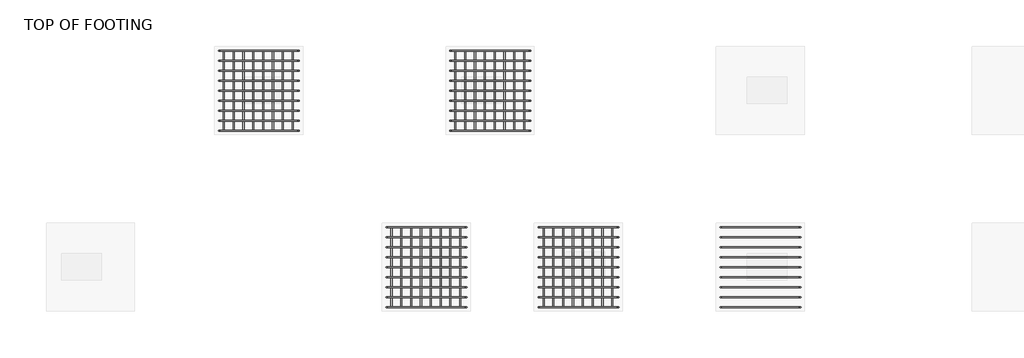
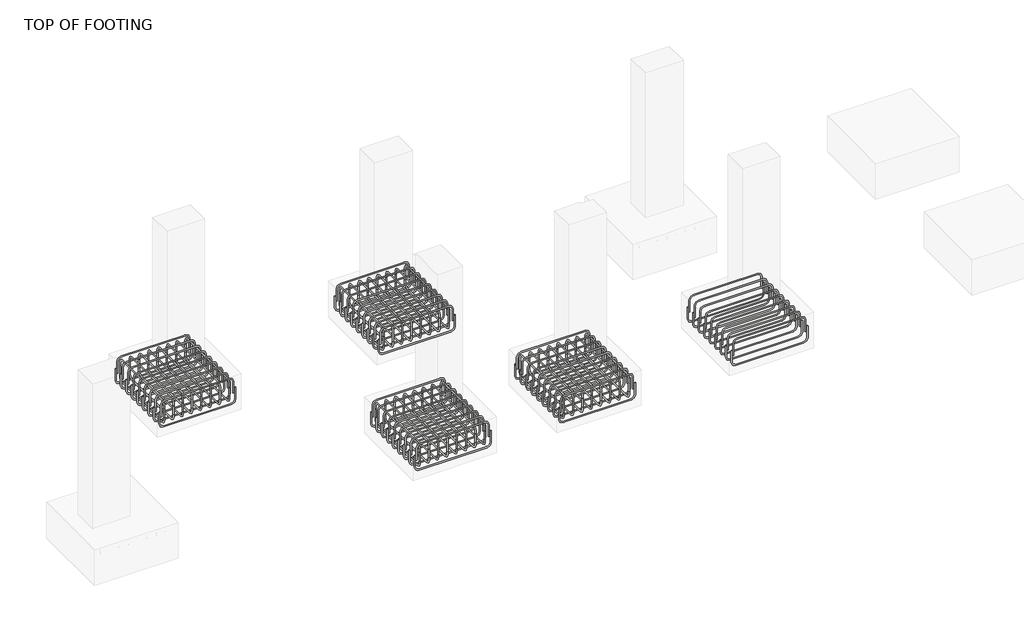
# One storey, part 7 of 20: 18 reinforcing bars.
"""IFC4 building model written with IfcOpenShell, lengths in millimetres."""

from ifc_helpers import new_model, si_unit, point, frame, origin, place, context, project, spatial, polyline, circle_curve, trimmed, segment, composite_curve, source, transform, mapped, element, save
from ifc_brep_helpers import swept_disk

model = new_model("IFC4")

# Units and contexts
model_context = context("Model", 3, world=origin())
ifc_project = project(units=[si_unit("LENGTHUNIT", "METRE", prefix="MILLI")], contexts=[model_context])

# Site, building, storey
site = spatial("IfcSite", under=ifc_project)
building = spatial("IfcBuilding", under=site)
storey = spatial("IfcBuildingStorey", under=building, Name="TOP OF FOOTING", Elevation=-1828.8)

# Reinforcing bars
placement = place(None, origin())
reinforcing_bar_shape = source(origin(), model_context, "Body", "SolidModel", [
    swept_disk(composite_curve([segment(polyline([(10322.7663908, -11304.2470059, -2006.6587682), (10322.7663908, -11304.2470059, -2153.9587682)]), True, "CONTINUOUS"), segment(trimmed(circle_curve(frame((10276.4163908, -11304.2470059, -2153.9587682), z_axis=(0.0, 1.0, 0.0), x_axis=(46.350000000000364, 0.0, 0.0)), 46.35), [point((10322.7663908, -11304.2470059, -2153.9587682))], [point((10276.4163908, -11304.2470059, -2200.3087682))], True, "CARTESIAN"), True, "CONTINUOUS"), segment(polyline([(10276.4163908, -11304.2470059, -2200.3087682), (9461.8163908, -11304.2470059, -2200.3087682)]), True, "CONTINUOUS"), segment(trimmed(circle_curve(frame((9461.8163908, -11304.2470059, -2153.9587682), z_axis=(0.0, 1.0, 0.0), x_axis=(0.0, 0.0, -46.34999999999991)), 46.35), [point((9461.8163908, -11304.2470059, -2200.3087682))], [point((9415.4663908, -11304.2470059, -2153.9587682))], True, "CARTESIAN"), True, "CONTINUOUS"), segment(polyline([(9415.4663908, -11304.2470059, -2153.9587682), (9415.4663908, -11304.2470059, -2006.6587682)]), True, "CONTINUOUS")], self_intersect=False), 6.35),
])
element("IfcReinforcingBar", 1, at=placement, inside=storey, context=model_context, shape_type="MappedRepresentation", body=[
    mapped(reinforcing_bar_shape, transform((0.0, 0.0, 0.0), x_axis=(1.0, 0.0, 0.0), y_axis=(0.0, 1.0, 0.0), z_axis=(0.0, 0.0, 1.0))),
    mapped(reinforcing_bar_shape, transform((0.0, -113.4125, 0.0), x_axis=(1.0, 0.0, 0.0), y_axis=(0.0, 1.0, 0.0), z_axis=(0.0, 0.0, 1.0))),
    mapped(reinforcing_bar_shape, transform((0.0, -226.825, 0.0), x_axis=(1.0, 0.0, 0.0), y_axis=(0.0, 1.0, 0.0), z_axis=(0.0, 0.0, 1.0))),
    mapped(reinforcing_bar_shape, transform((0.0, -340.2375, 0.0), x_axis=(1.0, 0.0, 0.0), y_axis=(0.0, 1.0, 0.0), z_axis=(0.0, 0.0, 1.0))),
    mapped(reinforcing_bar_shape, transform((0.0, -453.65, 0.0), x_axis=(1.0, 0.0, 0.0), y_axis=(0.0, 1.0, 0.0), z_axis=(0.0, 0.0, 1.0))),
    mapped(reinforcing_bar_shape, transform((0.0, -567.0625, 0.0), x_axis=(1.0, 0.0, 0.0), y_axis=(0.0, 1.0, 0.0), z_axis=(0.0, 0.0, 1.0))),
    mapped(reinforcing_bar_shape, transform((0.0, -680.475, 0.0), x_axis=(1.0, 0.0, 0.0), y_axis=(0.0, 1.0, 0.0), z_axis=(0.0, 0.0, 1.0))),
    mapped(reinforcing_bar_shape, transform((0.0, -793.8875, 0.0), x_axis=(1.0, 0.0, 0.0), y_axis=(0.0, 1.0, 0.0), z_axis=(0.0, 0.0, 1.0))),
    mapped(reinforcing_bar_shape, transform((0.0, -907.3, 0.0), x_axis=(1.0, 0.0, 0.0), y_axis=(0.0, 1.0, 0.0), z_axis=(0.0, 0.0, 1.0))),
])
reinforcing_bar_2_shape = source(origin(), model_context, "Body", "SolidModel", [
    swept_disk(composite_curve([segment(polyline([(9434.9405021, -11304.2470059, -2068.8), (9434.9405021, -11304.2470059, -1921.5)]), True, "CONTINUOUS"), segment(trimmed(circle_curve(frame((9481.2905021, -11304.2470059, -1921.5), z_axis=(0.0, 1.0, 0.0), x_axis=(-46.350000000000364, 0.0, 0.0)), 46.35), [point((9434.9405021, -11304.2470059, -1921.5))], [point((9481.2905021, -11304.2470059, -1875.15))], True, "CARTESIAN"), True, "CONTINUOUS"), segment(polyline([(9481.2905021, -11304.2470059, -1875.15), (10250.7539017, -11304.2470059, -1875.15)]), True, "CONTINUOUS"), segment(trimmed(circle_curve(frame((10250.7539017, -11304.2470059, -1921.5), z_axis=(0.0, 1.0, 0.0), x_axis=(0.0, 0.0, 46.34999999999991)), 46.35), [point((10250.7539017, -11304.2470059, -1875.15))], [point((10297.1039017, -11304.2470059, -1921.5))], True, "CARTESIAN"), True, "CONTINUOUS"), segment(polyline([(10297.1039017, -11304.2470059, -1921.5), (10297.1039017, -11304.2470059, -2068.8)]), True, "CONTINUOUS")], self_intersect=False), 6.35),
])
element("IfcReinforcingBar", 2, at=placement, inside=storey, context=model_context, shape_type="MappedRepresentation", body=[
    mapped(reinforcing_bar_2_shape, transform((0.0, 0.0, 0.0), x_axis=(1.0, 0.0, 0.0), y_axis=(0.0, 1.0, 0.0), z_axis=(0.0, 0.0, 1.0))),
    mapped(reinforcing_bar_2_shape, transform((0.0, -113.4125, 0.0), x_axis=(1.0, 0.0, 0.0), y_axis=(0.0, 1.0, 0.0), z_axis=(0.0, 0.0, 1.0))),
    mapped(reinforcing_bar_2_shape, transform((0.0, -226.825, 0.0), x_axis=(1.0, 0.0, 0.0), y_axis=(0.0, 1.0, 0.0), z_axis=(0.0, 0.0, 1.0))),
    mapped(reinforcing_bar_2_shape, transform((0.0, -340.2375, 0.0), x_axis=(1.0, 0.0, 0.0), y_axis=(0.0, 1.0, 0.0), z_axis=(0.0, 0.0, 1.0))),
    mapped(reinforcing_bar_2_shape, transform((0.0, -453.65, 0.0), x_axis=(1.0, 0.0, 0.0), y_axis=(0.0, 1.0, 0.0), z_axis=(0.0, 0.0, 1.0))),
    mapped(reinforcing_bar_2_shape, transform((0.0, -567.0625, 0.0), x_axis=(1.0, 0.0, 0.0), y_axis=(0.0, 1.0, 0.0), z_axis=(0.0, 0.0, 1.0))),
    mapped(reinforcing_bar_2_shape, transform((0.0, -680.475, 0.0), x_axis=(1.0, 0.0, 0.0), y_axis=(0.0, 1.0, 0.0), z_axis=(0.0, 0.0, 1.0))),
    mapped(reinforcing_bar_2_shape, transform((0.0, -793.8875, 0.0), x_axis=(1.0, 0.0, 0.0), y_axis=(0.0, 1.0, 0.0), z_axis=(0.0, 0.0, 1.0))),
    mapped(reinforcing_bar_2_shape, transform((0.0, -907.3, 0.0), x_axis=(1.0, 0.0, 0.0), y_axis=(0.0, 1.0, 0.0), z_axis=(0.0, 0.0, 1.0))),
])
reinforcing_bar_3_shape = source(origin(), model_context, "Body", "SolidModel", [
    swept_disk(composite_curve([segment(polyline([(7260.5179014, -9303.4578267, -2006.6587682), (7260.5179014, -9303.4578267, -2153.9587682)]), True, "CONTINUOUS"), segment(trimmed(circle_curve(frame((7214.1679014, -9303.4578267, -2153.9587682), z_axis=(0.0, 1.0, 0.0), x_axis=(46.349999999999454, 0.0, 0.0)), 46.35), [point((7260.5179014, -9303.4578267, -2153.9587682))], [point((7214.1679014, -9303.4578267, -2200.3087682))], True, "CARTESIAN"), True, "CONTINUOUS"), segment(polyline([(7214.1679014, -9303.4578267, -2200.3087682), (6399.5679014, -9303.4578267, -2200.3087682)]), True, "CONTINUOUS"), segment(trimmed(circle_curve(frame((6399.5679014, -9303.4578267, -2153.9587682), z_axis=(0.0, 1.0, 0.0), x_axis=(0.0, 0.0, -46.34999999999991)), 46.35), [point((6399.5679014, -9303.4578267, -2200.3087682))], [point((6353.2179014, -9303.4578267, -2153.9587682))], True, "CARTESIAN"), True, "CONTINUOUS"), segment(polyline([(6353.2179014, -9303.4578267, -2153.9587682), (6353.2179014, -9303.4578267, -2006.6587682)]), True, "CONTINUOUS")], self_intersect=False), 6.35),
])
element("IfcReinforcingBar", 3, at=placement, inside=storey, context=model_context, shape_type="MappedRepresentation", body=[
    mapped(reinforcing_bar_3_shape, transform((0.0, 0.0, 0.0), x_axis=(1.0, 0.0, 0.0), y_axis=(0.0, 1.0, 0.0), z_axis=(0.0, 0.0, 1.0))),
    mapped(reinforcing_bar_3_shape, transform((0.0, -113.4125, 0.0), x_axis=(1.0, 0.0, 0.0), y_axis=(0.0, 1.0, 0.0), z_axis=(0.0, 0.0, 1.0))),
    mapped(reinforcing_bar_3_shape, transform((0.0, -226.825, 0.0), x_axis=(1.0, 0.0, 0.0), y_axis=(0.0, 1.0, 0.0), z_axis=(0.0, 0.0, 1.0))),
    mapped(reinforcing_bar_3_shape, transform((0.0, -340.2375, 0.0), x_axis=(1.0, 0.0, 0.0), y_axis=(0.0, 1.0, 0.0), z_axis=(0.0, 0.0, 1.0))),
    mapped(reinforcing_bar_3_shape, transform((0.0, -453.65, 0.0), x_axis=(1.0, 0.0, 0.0), y_axis=(0.0, 1.0, 0.0), z_axis=(0.0, 0.0, 1.0))),
    mapped(reinforcing_bar_3_shape, transform((0.0, -567.0625, 0.0), x_axis=(1.0, 0.0, 0.0), y_axis=(0.0, 1.0, 0.0), z_axis=(0.0, 0.0, 1.0))),
    mapped(reinforcing_bar_3_shape, transform((0.0, -680.475, 0.0), x_axis=(1.0, 0.0, 0.0), y_axis=(0.0, 1.0, 0.0), z_axis=(0.0, 0.0, 1.0))),
    mapped(reinforcing_bar_3_shape, transform((0.0, -793.8875, 0.0), x_axis=(1.0, 0.0, 0.0), y_axis=(0.0, 1.0, 0.0), z_axis=(0.0, 0.0, 1.0))),
    mapped(reinforcing_bar_3_shape, transform((0.0, -907.3, 0.0), x_axis=(1.0, 0.0, 0.0), y_axis=(0.0, 1.0, 0.0), z_axis=(0.0, 0.0, 1.0))),
])
reinforcing_bar_4_shape = source(origin(), model_context, "Body", "SolidModel", [
    swept_disk(composite_curve([segment(polyline([(6372.6920127, -9303.4578267, -2068.8), (6372.6920127, -9303.4578267, -1921.5)]), True, "CONTINUOUS"), segment(trimmed(circle_curve(frame((6419.0420127, -9303.4578267, -1921.5), z_axis=(0.0, 1.0, 0.0), x_axis=(-46.349999999999454, 0.0, 0.0)), 46.35), [point((6372.6920127, -9303.4578267, -1921.5))], [point((6419.0420127, -9303.4578267, -1875.15))], True, "CARTESIAN"), True, "CONTINUOUS"), segment(polyline([(6419.0420127, -9303.4578267, -1875.15), (7188.5054124, -9303.4578267, -1875.15)]), True, "CONTINUOUS"), segment(trimmed(circle_curve(frame((7188.5054124, -9303.4578267, -1921.5), z_axis=(0.0, 1.0, 0.0), x_axis=(0.0, 0.0, 46.34999999999991)), 46.35), [point((7188.5054124, -9303.4578267, -1875.15))], [point((7234.8554124, -9303.4578267, -1921.5))], True, "CARTESIAN"), True, "CONTINUOUS"), segment(polyline([(7234.8554124, -9303.4578267, -1921.5), (7234.8554124, -9303.4578267, -2068.8)]), True, "CONTINUOUS")], self_intersect=False), 6.35),
])
element("IfcReinforcingBar", 4, at=placement, inside=storey, context=model_context, shape_type="MappedRepresentation", body=[
    mapped(reinforcing_bar_4_shape, transform((0.0, 0.0, 0.0), x_axis=(1.0, 0.0, 0.0), y_axis=(0.0, 1.0, 0.0), z_axis=(0.0, 0.0, 1.0))),
    mapped(reinforcing_bar_4_shape, transform((0.0, -113.4125, 0.0), x_axis=(1.0, 0.0, 0.0), y_axis=(0.0, 1.0, 0.0), z_axis=(0.0, 0.0, 1.0))),
    mapped(reinforcing_bar_4_shape, transform((0.0, -226.825, 0.0), x_axis=(1.0, 0.0, 0.0), y_axis=(0.0, 1.0, 0.0), z_axis=(0.0, 0.0, 1.0))),
    mapped(reinforcing_bar_4_shape, transform((0.0, -340.2375, 0.0), x_axis=(1.0, 0.0, 0.0), y_axis=(0.0, 1.0, 0.0), z_axis=(0.0, 0.0, 1.0))),
    mapped(reinforcing_bar_4_shape, transform((0.0, -453.65, 0.0), x_axis=(1.0, 0.0, 0.0), y_axis=(0.0, 1.0, 0.0), z_axis=(0.0, 0.0, 1.0))),
    mapped(reinforcing_bar_4_shape, transform((0.0, -567.0625, 0.0), x_axis=(1.0, 0.0, 0.0), y_axis=(0.0, 1.0, 0.0), z_axis=(0.0, 0.0, 1.0))),
    mapped(reinforcing_bar_4_shape, transform((0.0, -680.475, 0.0), x_axis=(1.0, 0.0, 0.0), y_axis=(0.0, 1.0, 0.0), z_axis=(0.0, 0.0, 1.0))),
    mapped(reinforcing_bar_4_shape, transform((0.0, -793.8875, 0.0), x_axis=(1.0, 0.0, 0.0), y_axis=(0.0, 1.0, 0.0), z_axis=(0.0, 0.0, 1.0))),
    mapped(reinforcing_bar_4_shape, transform((0.0, -907.3, 0.0), x_axis=(1.0, 0.0, 0.0), y_axis=(0.0, 1.0, 0.0), z_axis=(0.0, 0.0, 1.0))),
])
reinforcing_bar_5_shape = source(origin(), model_context, "Body", "SolidModel", [
    swept_disk(composite_curve([segment(polyline([(7189.02094, -9303.4578267, -2086.1951968), (7189.02094, -9303.4578267, -1938.8951968)]), True, "CONTINUOUS"), segment(trimmed(circle_curve(frame((7189.02094, -9349.8078267, -1938.8951968), z_axis=(1.0, 0.0, 0.0), x_axis=(0.0, 46.350000000000364, 0.0)), 46.35), [point((7189.02094, -9303.4578267, -1938.8951968))], [point((7189.02094, -9349.8078267, -1892.5451968))], True, "CARTESIAN"), True, "CONTINUOUS"), segment(polyline([(7189.02094, -9349.8078267, -1892.5451968), (7189.02094, -10164.4078267, -1892.5451968)]), True, "CONTINUOUS"), segment(trimmed(circle_curve(frame((7189.02094, -10164.4078267, -1938.8951968), z_axis=(1.0, 0.0, 0.0), x_axis=(0.0, 0.0, 46.34999999999991)), 46.35), [point((7189.02094, -10164.4078267, -1892.5451968))], [point((7189.02094, -10210.7578267, -1938.8951968))], True, "CARTESIAN"), True, "CONTINUOUS"), segment(polyline([(7189.02094, -10210.7578267, -1938.8951968), (7189.02094, -10210.7578267, -2086.1951968)]), True, "CONTINUOUS")], self_intersect=False), 6.35),
])
element("IfcReinforcingBar", 5, at=placement, inside=storey, context=model_context, shape_type="MappedRepresentation", body=[
    mapped(reinforcing_bar_5_shape, transform((0.0, 0.0, 0.0), x_axis=(1.0, 0.0, 0.0), y_axis=(0.0, 1.0, 0.0), z_axis=(0.0, 0.0, 1.0))),
    mapped(reinforcing_bar_5_shape, transform((-111.2862402, 0.0, 0.0), x_axis=(1.0, 0.0, 0.0), y_axis=(0.0, 1.0, 0.0), z_axis=(0.0, 0.0, 1.0))),
    mapped(reinforcing_bar_5_shape, transform((-222.5724804, 0.0, 0.0), x_axis=(1.0, 0.0, 0.0), y_axis=(0.0, 1.0, 0.0), z_axis=(0.0, 0.0, 1.0))),
    mapped(reinforcing_bar_5_shape, transform((-333.8587205, 0.0, 0.0), x_axis=(1.0, 0.0, 0.0), y_axis=(0.0, 1.0, 0.0), z_axis=(0.0, 0.0, 1.0))),
    mapped(reinforcing_bar_5_shape, transform((-445.1449607, 0.0, 0.0), x_axis=(1.0, 0.0, 0.0), y_axis=(0.0, 1.0, 0.0), z_axis=(0.0, 0.0, 1.0))),
    mapped(reinforcing_bar_5_shape, transform((-556.4312009, 0.0, 0.0), x_axis=(1.0, 0.0, 0.0), y_axis=(0.0, 1.0, 0.0), z_axis=(0.0, 0.0, 1.0))),
    mapped(reinforcing_bar_5_shape, transform((-667.7174411, 0.0, 0.0), x_axis=(1.0, 0.0, 0.0), y_axis=(0.0, 1.0, 0.0), z_axis=(0.0, 0.0, 1.0))),
    mapped(reinforcing_bar_5_shape, transform((-779.0036813, 0.0, 0.0), x_axis=(1.0, 0.0, 0.0), y_axis=(0.0, 1.0, 0.0), z_axis=(0.0, 0.0, 1.0))),
])
reinforcing_bar_6_shape = source(origin(), model_context, "Body", "SolidModel", [
    swept_disk(composite_curve([segment(polyline([(6410.0172587, -9303.4578267, -1979.1645013), (6410.0172587, -9303.4578267, -2126.4645013)]), True, "CONTINUOUS"), segment(trimmed(circle_curve(frame((6410.0172587, -9349.8078267, -2126.4645013), z_axis=(-1.0, 0.0, 0.0), x_axis=(0.0, 46.350000000000364, 0.0)), 46.35), [point((6410.0172587, -9303.4578267, -2126.4645013))], [point((6410.0172587, -9349.8078267, -2172.8145013))], True, "CARTESIAN"), True, "CONTINUOUS"), segment(polyline([(6410.0172587, -9349.8078267, -2172.8145013), (6410.0172587, -10164.4078267, -2172.8145013)]), True, "CONTINUOUS"), segment(trimmed(circle_curve(frame((6410.0172587, -10164.4078267, -2126.4645013), z_axis=(-1.0, 0.0, 0.0), x_axis=(0.0, 0.0, -46.34999999999991)), 46.35), [point((6410.0172587, -10164.4078267, -2172.8145013))], [point((6410.0172587, -10210.7578267, -2126.4645013))], True, "CARTESIAN"), True, "CONTINUOUS"), segment(polyline([(6410.0172587, -10210.7578267, -2126.4645013), (6410.0172587, -10210.7578267, -1979.1645013)]), True, "CONTINUOUS")], self_intersect=False), 6.35),
])
element("IfcReinforcingBar", 6, at=placement, inside=storey, context=model_context, shape_type="MappedRepresentation", body=[
    mapped(reinforcing_bar_6_shape, transform((0.0, 0.0, 0.0), x_axis=(1.0, 0.0, 0.0), y_axis=(0.0, 1.0, 0.0), z_axis=(0.0, 0.0, 1.0))),
    mapped(reinforcing_bar_6_shape, transform((111.2862402, 0.0, 0.0), x_axis=(1.0, 0.0, 0.0), y_axis=(0.0, 1.0, 0.0), z_axis=(0.0, 0.0, 1.0))),
    mapped(reinforcing_bar_6_shape, transform((222.5724804, 0.0, 0.0), x_axis=(1.0, 0.0, 0.0), y_axis=(0.0, 1.0, 0.0), z_axis=(0.0, 0.0, 1.0))),
    mapped(reinforcing_bar_6_shape, transform((333.8587205, 0.0, 0.0), x_axis=(1.0, 0.0, 0.0), y_axis=(0.0, 1.0, 0.0), z_axis=(0.0, 0.0, 1.0))),
    mapped(reinforcing_bar_6_shape, transform((445.1449607, 0.0, 0.0), x_axis=(1.0, 0.0, 0.0), y_axis=(0.0, 1.0, 0.0), z_axis=(0.0, 0.0, 1.0))),
    mapped(reinforcing_bar_6_shape, transform((556.4312009, 0.0, 0.0), x_axis=(1.0, 0.0, 0.0), y_axis=(0.0, 1.0, 0.0), z_axis=(0.0, 0.0, 1.0))),
    mapped(reinforcing_bar_6_shape, transform((667.7174411, 0.0, 0.0), x_axis=(1.0, 0.0, 0.0), y_axis=(0.0, 1.0, 0.0), z_axis=(0.0, 0.0, 1.0))),
    mapped(reinforcing_bar_6_shape, transform((779.0036813, 0.0, 0.0), x_axis=(1.0, 0.0, 0.0), y_axis=(0.0, 1.0, 0.0), z_axis=(0.0, 0.0, 1.0))),
])
reinforcing_bar_7_shape = source(origin(), model_context, "Body", "SolidModel", [
    swept_disk(composite_curve([segment(polyline([(6536.1748054, -11304.2470059, -2006.6587682), (6536.1748054, -11304.2470059, -2153.9587682)]), True, "CONTINUOUS"), segment(trimmed(circle_curve(frame((6489.8248054, -11304.2470059, -2153.9587682), z_axis=(0.0, 1.0, 0.0), x_axis=(46.350000000000364, 0.0, 0.0)), 46.35), [point((6536.1748054, -11304.2470059, -2153.9587682))], [point((6489.8248054, -11304.2470059, -2200.3087682))], True, "CARTESIAN"), True, "CONTINUOUS"), segment(polyline([(6489.8248054, -11304.2470059, -2200.3087682), (5675.2248054, -11304.2470059, -2200.3087682)]), True, "CONTINUOUS"), segment(trimmed(circle_curve(frame((5675.2248054, -11304.2470059, -2153.9587682), z_axis=(0.0, 1.0, 0.0), x_axis=(0.0, 0.0, -46.34999999999991)), 46.35), [point((5675.2248054, -11304.2470059, -2200.3087682))], [point((5628.8748054, -11304.2470059, -2153.9587682))], True, "CARTESIAN"), True, "CONTINUOUS"), segment(polyline([(5628.8748054, -11304.2470059, -2153.9587682), (5628.8748054, -11304.2470059, -2006.6587682)]), True, "CONTINUOUS")], self_intersect=False), 6.35),
])
element("IfcReinforcingBar", 7, at=placement, inside=storey, context=model_context, shape_type="MappedRepresentation", body=[
    mapped(reinforcing_bar_7_shape, transform((0.0, 0.0, 0.0), x_axis=(1.0, 0.0, 0.0), y_axis=(0.0, 1.0, 0.0), z_axis=(0.0, 0.0, 1.0))),
    mapped(reinforcing_bar_7_shape, transform((0.0, -113.4125, 0.0), x_axis=(1.0, 0.0, 0.0), y_axis=(0.0, 1.0, 0.0), z_axis=(0.0, 0.0, 1.0))),
    mapped(reinforcing_bar_7_shape, transform((0.0, -226.825, 0.0), x_axis=(1.0, 0.0, 0.0), y_axis=(0.0, 1.0, 0.0), z_axis=(0.0, 0.0, 1.0))),
    mapped(reinforcing_bar_7_shape, transform((0.0, -340.2375, 0.0), x_axis=(1.0, 0.0, 0.0), y_axis=(0.0, 1.0, 0.0), z_axis=(0.0, 0.0, 1.0))),
    mapped(reinforcing_bar_7_shape, transform((0.0, -453.65, 0.0), x_axis=(1.0, 0.0, 0.0), y_axis=(0.0, 1.0, 0.0), z_axis=(0.0, 0.0, 1.0))),
    mapped(reinforcing_bar_7_shape, transform((0.0, -567.0625, 0.0), x_axis=(1.0, 0.0, 0.0), y_axis=(0.0, 1.0, 0.0), z_axis=(0.0, 0.0, 1.0))),
    mapped(reinforcing_bar_7_shape, transform((0.0, -680.475, 0.0), x_axis=(1.0, 0.0, 0.0), y_axis=(0.0, 1.0, 0.0), z_axis=(0.0, 0.0, 1.0))),
    mapped(reinforcing_bar_7_shape, transform((0.0, -793.8875, 0.0), x_axis=(1.0, 0.0, 0.0), y_axis=(0.0, 1.0, 0.0), z_axis=(0.0, 0.0, 1.0))),
    mapped(reinforcing_bar_7_shape, transform((0.0, -907.3, 0.0), x_axis=(1.0, 0.0, 0.0), y_axis=(0.0, 1.0, 0.0), z_axis=(0.0, 0.0, 1.0))),
])
reinforcing_bar_8_shape = source(origin(), model_context, "Body", "SolidModel", [
    swept_disk(composite_curve([segment(polyline([(5648.3489167, -11304.2470059, -2068.8), (5648.3489167, -11304.2470059, -1921.5)]), True, "CONTINUOUS"), segment(trimmed(circle_curve(frame((5694.6989167, -11304.2470059, -1921.5), z_axis=(0.0, 1.0, 0.0), x_axis=(-46.350000000000364, 0.0, 0.0)), 46.35), [point((5648.3489167, -11304.2470059, -1921.5))], [point((5694.6989167, -11304.2470059, -1875.15))], True, "CARTESIAN"), True, "CONTINUOUS"), segment(polyline([(5694.6989167, -11304.2470059, -1875.15), (6464.1623164, -11304.2470059, -1875.15)]), True, "CONTINUOUS"), segment(trimmed(circle_curve(frame((6464.1623164, -11304.2470059, -1921.5), z_axis=(0.0, 1.0, 0.0), x_axis=(0.0, 0.0, 46.34999999999991)), 46.35), [point((6464.1623164, -11304.2470059, -1875.15))], [point((6510.5123164, -11304.2470059, -1921.5))], True, "CARTESIAN"), True, "CONTINUOUS"), segment(polyline([(6510.5123164, -11304.2470059, -1921.5), (6510.5123164, -11304.2470059, -2068.8)]), True, "CONTINUOUS")], self_intersect=False), 6.35),
])
element("IfcReinforcingBar", 8, at=placement, inside=storey, context=model_context, shape_type="MappedRepresentation", body=[
    mapped(reinforcing_bar_8_shape, transform((0.0, 0.0, 0.0), x_axis=(1.0, 0.0, 0.0), y_axis=(0.0, 1.0, 0.0), z_axis=(0.0, 0.0, 1.0))),
    mapped(reinforcing_bar_8_shape, transform((0.0, -113.4125, 0.0), x_axis=(1.0, 0.0, 0.0), y_axis=(0.0, 1.0, 0.0), z_axis=(0.0, 0.0, 1.0))),
    mapped(reinforcing_bar_8_shape, transform((0.0, -226.825, 0.0), x_axis=(1.0, 0.0, 0.0), y_axis=(0.0, 1.0, 0.0), z_axis=(0.0, 0.0, 1.0))),
    mapped(reinforcing_bar_8_shape, transform((0.0, -340.2375, 0.0), x_axis=(1.0, 0.0, 0.0), y_axis=(0.0, 1.0, 0.0), z_axis=(0.0, 0.0, 1.0))),
    mapped(reinforcing_bar_8_shape, transform((0.0, -453.65, 0.0), x_axis=(1.0, 0.0, 0.0), y_axis=(0.0, 1.0, 0.0), z_axis=(0.0, 0.0, 1.0))),
    mapped(reinforcing_bar_8_shape, transform((0.0, -567.0625, 0.0), x_axis=(1.0, 0.0, 0.0), y_axis=(0.0, 1.0, 0.0), z_axis=(0.0, 0.0, 1.0))),
    mapped(reinforcing_bar_8_shape, transform((0.0, -680.475, 0.0), x_axis=(1.0, 0.0, 0.0), y_axis=(0.0, 1.0, 0.0), z_axis=(0.0, 0.0, 1.0))),
    mapped(reinforcing_bar_8_shape, transform((0.0, -793.8875, 0.0), x_axis=(1.0, 0.0, 0.0), y_axis=(0.0, 1.0, 0.0), z_axis=(0.0, 0.0, 1.0))),
    mapped(reinforcing_bar_8_shape, transform((0.0, -907.3, 0.0), x_axis=(1.0, 0.0, 0.0), y_axis=(0.0, 1.0, 0.0), z_axis=(0.0, 0.0, 1.0))),
])
reinforcing_bar_9_shape = source(origin(), model_context, "Body", "SolidModel", [
    swept_disk(composite_curve([segment(polyline([(6464.677844, -11304.2470059, -2086.1951968), (6464.677844, -11304.2470059, -1938.8951968)]), True, "CONTINUOUS"), segment(trimmed(circle_curve(frame((6464.677844, -11350.5970059, -1938.8951968), z_axis=(1.0, 0.0, 0.0), x_axis=(0.0, 46.349999999998545, 0.0)), 46.35), [point((6464.677844, -11304.2470059, -1938.8951968))], [point((6464.677844, -11350.5970059, -1892.5451968))], True, "CARTESIAN"), True, "CONTINUOUS"), segment(polyline([(6464.677844, -11350.5970059, -1892.5451968), (6464.677844, -12165.1970059, -1892.5451968)]), True, "CONTINUOUS"), segment(trimmed(circle_curve(frame((6464.677844, -12165.1970059, -1938.8951968), z_axis=(1.0, 0.0, 0.0), x_axis=(0.0, 0.0, 46.34999999999991)), 46.35), [point((6464.677844, -12165.1970059, -1892.5451968))], [point((6464.677844, -12211.5470059, -1938.8951968))], True, "CARTESIAN"), True, "CONTINUOUS"), segment(polyline([(6464.677844, -12211.5470059, -1938.8951968), (6464.677844, -12211.5470059, -2086.1951968)]), True, "CONTINUOUS")], self_intersect=False), 6.35),
])
element("IfcReinforcingBar", 9, at=placement, inside=storey, context=model_context, shape_type="MappedRepresentation", body=[
    mapped(reinforcing_bar_9_shape, transform((0.0, 0.0, 0.0), x_axis=(1.0, 0.0, 0.0), y_axis=(0.0, 1.0, 0.0), z_axis=(0.0, 0.0, 1.0))),
    mapped(reinforcing_bar_9_shape, transform((-111.2862402, 0.0, 0.0), x_axis=(1.0, 0.0, 0.0), y_axis=(0.0, 1.0, 0.0), z_axis=(0.0, 0.0, 1.0))),
    mapped(reinforcing_bar_9_shape, transform((-222.5724804, 0.0, 0.0), x_axis=(1.0, 0.0, 0.0), y_axis=(0.0, 1.0, 0.0), z_axis=(0.0, 0.0, 1.0))),
    mapped(reinforcing_bar_9_shape, transform((-333.8587205, 0.0, 0.0), x_axis=(1.0, 0.0, 0.0), y_axis=(0.0, 1.0, 0.0), z_axis=(0.0, 0.0, 1.0))),
    mapped(reinforcing_bar_9_shape, transform((-445.1449607, 0.0, 0.0), x_axis=(1.0, 0.0, 0.0), y_axis=(0.0, 1.0, 0.0), z_axis=(0.0, 0.0, 1.0))),
    mapped(reinforcing_bar_9_shape, transform((-556.4312009, 0.0, 0.0), x_axis=(1.0, 0.0, 0.0), y_axis=(0.0, 1.0, 0.0), z_axis=(0.0, 0.0, 1.0))),
    mapped(reinforcing_bar_9_shape, transform((-667.7174411, 0.0, 0.0), x_axis=(1.0, 0.0, 0.0), y_axis=(0.0, 1.0, 0.0), z_axis=(0.0, 0.0, 1.0))),
    mapped(reinforcing_bar_9_shape, transform((-779.0036813, 0.0, 0.0), x_axis=(1.0, 0.0, 0.0), y_axis=(0.0, 1.0, 0.0), z_axis=(0.0, 0.0, 1.0))),
])
reinforcing_bar_10_shape = source(origin(), model_context, "Body", "SolidModel", [
    swept_disk(composite_curve([segment(polyline([(5685.6741627, -11304.2470059, -1979.1645013), (5685.6741627, -11304.2470059, -2126.4645013)]), True, "CONTINUOUS"), segment(trimmed(circle_curve(frame((5685.6741627, -11350.5970059, -2126.4645013), z_axis=(-1.0, 0.0, 0.0), x_axis=(0.0, 46.349999999998545, 0.0)), 46.35), [point((5685.6741627, -11304.2470059, -2126.4645013))], [point((5685.6741627, -11350.5970059, -2172.8145013))], True, "CARTESIAN"), True, "CONTINUOUS"), segment(polyline([(5685.6741627, -11350.5970059, -2172.8145013), (5685.6741627, -12165.1970059, -2172.8145013)]), True, "CONTINUOUS"), segment(trimmed(circle_curve(frame((5685.6741627, -12165.1970059, -2126.4645013), z_axis=(-1.0, 0.0, 0.0), x_axis=(0.0, 0.0, -46.34999999999991)), 46.35), [point((5685.6741627, -12165.1970059, -2172.8145013))], [point((5685.6741627, -12211.5470059, -2126.4645013))], True, "CARTESIAN"), True, "CONTINUOUS"), segment(polyline([(5685.6741627, -12211.5470059, -2126.4645013), (5685.6741627, -12211.5470059, -1979.1645013)]), True, "CONTINUOUS")], self_intersect=False), 6.35),
])
element("IfcReinforcingBar", 10, at=placement, inside=storey, context=model_context, shape_type="MappedRepresentation", body=[
    mapped(reinforcing_bar_10_shape, transform((0.0, 0.0, 0.0), x_axis=(1.0, 0.0, 0.0), y_axis=(0.0, 1.0, 0.0), z_axis=(0.0, 0.0, 1.0))),
    mapped(reinforcing_bar_10_shape, transform((111.2862402, 0.0, 0.0), x_axis=(1.0, 0.0, 0.0), y_axis=(0.0, 1.0, 0.0), z_axis=(0.0, 0.0, 1.0))),
    mapped(reinforcing_bar_10_shape, transform((222.5724804, 0.0, 0.0), x_axis=(1.0, 0.0, 0.0), y_axis=(0.0, 1.0, 0.0), z_axis=(0.0, 0.0, 1.0))),
    mapped(reinforcing_bar_10_shape, transform((333.8587205, 0.0, 0.0), x_axis=(1.0, 0.0, 0.0), y_axis=(0.0, 1.0, 0.0), z_axis=(0.0, 0.0, 1.0))),
    mapped(reinforcing_bar_10_shape, transform((445.1449607, 0.0, 0.0), x_axis=(1.0, 0.0, 0.0), y_axis=(0.0, 1.0, 0.0), z_axis=(0.0, 0.0, 1.0))),
    mapped(reinforcing_bar_10_shape, transform((556.4312009, 0.0, 0.0), x_axis=(1.0, 0.0, 0.0), y_axis=(0.0, 1.0, 0.0), z_axis=(0.0, 0.0, 1.0))),
    mapped(reinforcing_bar_10_shape, transform((667.7174411, 0.0, 0.0), x_axis=(1.0, 0.0, 0.0), y_axis=(0.0, 1.0, 0.0), z_axis=(0.0, 0.0, 1.0))),
    mapped(reinforcing_bar_10_shape, transform((779.0036813, 0.0, 0.0), x_axis=(1.0, 0.0, 0.0), y_axis=(0.0, 1.0, 0.0), z_axis=(0.0, 0.0, 1.0))),
])
reinforcing_bar_11_shape = source(origin(), model_context, "Body", "SolidModel", [
    swept_disk(composite_curve([segment(polyline([(8260.5179014, -11304.2470059, -2006.6587682), (8260.5179014, -11304.2470059, -2153.9587682)]), True, "CONTINUOUS"), segment(trimmed(circle_curve(frame((8214.1679014, -11304.2470059, -2153.9587682), z_axis=(0.0, 1.0, 0.0), x_axis=(46.350000000000364, 0.0, 0.0)), 46.35), [point((8260.5179014, -11304.2470059, -2153.9587682))], [point((8214.1679014, -11304.2470059, -2200.3087682))], True, "CARTESIAN"), True, "CONTINUOUS"), segment(polyline([(8214.1679014, -11304.2470059, -2200.3087682), (7399.5679014, -11304.2470059, -2200.3087682)]), True, "CONTINUOUS"), segment(trimmed(circle_curve(frame((7399.5679014, -11304.2470059, -2153.9587682), z_axis=(0.0, 1.0, 0.0), x_axis=(0.0, 0.0, -46.34999999999991)), 46.35), [point((7399.5679014, -11304.2470059, -2200.3087682))], [point((7353.2179014, -11304.2470059, -2153.9587682))], True, "CARTESIAN"), True, "CONTINUOUS"), segment(polyline([(7353.2179014, -11304.2470059, -2153.9587682), (7353.2179014, -11304.2470059, -2006.6587682)]), True, "CONTINUOUS")], self_intersect=False), 6.35),
])
element("IfcReinforcingBar", 11, at=placement, inside=storey, context=model_context, shape_type="MappedRepresentation", body=[
    mapped(reinforcing_bar_11_shape, transform((0.0, 0.0, 0.0), x_axis=(1.0, 0.0, 0.0), y_axis=(0.0, 1.0, 0.0), z_axis=(0.0, 0.0, 1.0))),
    mapped(reinforcing_bar_11_shape, transform((0.0, -113.4125, 0.0), x_axis=(1.0, 0.0, 0.0), y_axis=(0.0, 1.0, 0.0), z_axis=(0.0, 0.0, 1.0))),
    mapped(reinforcing_bar_11_shape, transform((0.0, -226.825, 0.0), x_axis=(1.0, 0.0, 0.0), y_axis=(0.0, 1.0, 0.0), z_axis=(0.0, 0.0, 1.0))),
    mapped(reinforcing_bar_11_shape, transform((0.0, -340.2375, 0.0), x_axis=(1.0, 0.0, 0.0), y_axis=(0.0, 1.0, 0.0), z_axis=(0.0, 0.0, 1.0))),
    mapped(reinforcing_bar_11_shape, transform((0.0, -453.65, 0.0), x_axis=(1.0, 0.0, 0.0), y_axis=(0.0, 1.0, 0.0), z_axis=(0.0, 0.0, 1.0))),
    mapped(reinforcing_bar_11_shape, transform((0.0, -567.0625, 0.0), x_axis=(1.0, 0.0, 0.0), y_axis=(0.0, 1.0, 0.0), z_axis=(0.0, 0.0, 1.0))),
    mapped(reinforcing_bar_11_shape, transform((0.0, -680.475, 0.0), x_axis=(1.0, 0.0, 0.0), y_axis=(0.0, 1.0, 0.0), z_axis=(0.0, 0.0, 1.0))),
    mapped(reinforcing_bar_11_shape, transform((0.0, -793.8875, 0.0), x_axis=(1.0, 0.0, 0.0), y_axis=(0.0, 1.0, 0.0), z_axis=(0.0, 0.0, 1.0))),
    mapped(reinforcing_bar_11_shape, transform((0.0, -907.3, 0.0), x_axis=(1.0, 0.0, 0.0), y_axis=(0.0, 1.0, 0.0), z_axis=(0.0, 0.0, 1.0))),
])
reinforcing_bar_12_shape = source(origin(), model_context, "Body", "SolidModel", [
    swept_disk(composite_curve([segment(polyline([(7372.6920127, -11304.2470059, -2068.8), (7372.6920127, -11304.2470059, -1921.5)]), True, "CONTINUOUS"), segment(trimmed(circle_curve(frame((7419.0420127, -11304.2470059, -1921.5), z_axis=(0.0, 1.0, 0.0), x_axis=(-46.349999999999454, 0.0, 0.0)), 46.35), [point((7372.6920127, -11304.2470059, -1921.5))], [point((7419.0420127, -11304.2470059, -1875.15))], True, "CARTESIAN"), True, "CONTINUOUS"), segment(polyline([(7419.0420127, -11304.2470059, -1875.15), (8188.5054124, -11304.2470059, -1875.15)]), True, "CONTINUOUS"), segment(trimmed(circle_curve(frame((8188.5054124, -11304.2470059, -1921.5), z_axis=(0.0, 1.0, 0.0), x_axis=(0.0, 0.0, 46.34999999999991)), 46.35), [point((8188.5054124, -11304.2470059, -1875.15))], [point((8234.8554124, -11304.2470059, -1921.5))], True, "CARTESIAN"), True, "CONTINUOUS"), segment(polyline([(8234.8554124, -11304.2470059, -1921.5), (8234.8554124, -11304.2470059, -2068.8)]), True, "CONTINUOUS")], self_intersect=False), 6.35),
])
element("IfcReinforcingBar", 12, at=placement, inside=storey, context=model_context, shape_type="MappedRepresentation", body=[
    mapped(reinforcing_bar_12_shape, transform((0.0, 0.0, 0.0), x_axis=(1.0, 0.0, 0.0), y_axis=(0.0, 1.0, 0.0), z_axis=(0.0, 0.0, 1.0))),
    mapped(reinforcing_bar_12_shape, transform((0.0, -113.4125, 0.0), x_axis=(1.0, 0.0, 0.0), y_axis=(0.0, 1.0, 0.0), z_axis=(0.0, 0.0, 1.0))),
    mapped(reinforcing_bar_12_shape, transform((0.0, -226.825, 0.0), x_axis=(1.0, 0.0, 0.0), y_axis=(0.0, 1.0, 0.0), z_axis=(0.0, 0.0, 1.0))),
    mapped(reinforcing_bar_12_shape, transform((0.0, -340.2375, 0.0), x_axis=(1.0, 0.0, 0.0), y_axis=(0.0, 1.0, 0.0), z_axis=(0.0, 0.0, 1.0))),
    mapped(reinforcing_bar_12_shape, transform((0.0, -453.65, 0.0), x_axis=(1.0, 0.0, 0.0), y_axis=(0.0, 1.0, 0.0), z_axis=(0.0, 0.0, 1.0))),
    mapped(reinforcing_bar_12_shape, transform((0.0, -567.0625, 0.0), x_axis=(1.0, 0.0, 0.0), y_axis=(0.0, 1.0, 0.0), z_axis=(0.0, 0.0, 1.0))),
    mapped(reinforcing_bar_12_shape, transform((0.0, -680.475, 0.0), x_axis=(1.0, 0.0, 0.0), y_axis=(0.0, 1.0, 0.0), z_axis=(0.0, 0.0, 1.0))),
    mapped(reinforcing_bar_12_shape, transform((0.0, -793.8875, 0.0), x_axis=(1.0, 0.0, 0.0), y_axis=(0.0, 1.0, 0.0), z_axis=(0.0, 0.0, 1.0))),
    mapped(reinforcing_bar_12_shape, transform((0.0, -907.3, 0.0), x_axis=(1.0, 0.0, 0.0), y_axis=(0.0, 1.0, 0.0), z_axis=(0.0, 0.0, 1.0))),
])
reinforcing_bar_13_shape = source(origin(), model_context, "Body", "SolidModel", [
    swept_disk(composite_curve([segment(polyline([(8189.02094, -11304.2470059, -2086.1951968), (8189.02094, -11304.2470059, -1938.8951968)]), True, "CONTINUOUS"), segment(trimmed(circle_curve(frame((8189.02094, -11350.5970059, -1938.8951968), z_axis=(1.0, 0.0, 0.0), x_axis=(0.0, 46.349999999998545, 0.0)), 46.35), [point((8189.02094, -11304.2470059, -1938.8951968))], [point((8189.02094, -11350.5970059, -1892.5451968))], True, "CARTESIAN"), True, "CONTINUOUS"), segment(polyline([(8189.02094, -11350.5970059, -1892.5451968), (8189.02094, -12165.1970059, -1892.5451968)]), True, "CONTINUOUS"), segment(trimmed(circle_curve(frame((8189.02094, -12165.1970059, -1938.8951968), z_axis=(1.0, 0.0, 0.0), x_axis=(0.0, 0.0, 46.34999999999991)), 46.35), [point((8189.02094, -12165.1970059, -1892.5451968))], [point((8189.02094, -12211.5470059, -1938.8951968))], True, "CARTESIAN"), True, "CONTINUOUS"), segment(polyline([(8189.02094, -12211.5470059, -1938.8951968), (8189.02094, -12211.5470059, -2086.1951968)]), True, "CONTINUOUS")], self_intersect=False), 6.35),
])
element("IfcReinforcingBar", 13, at=placement, inside=storey, context=model_context, shape_type="MappedRepresentation", body=[
    mapped(reinforcing_bar_13_shape, transform((0.0, 0.0, 0.0), x_axis=(1.0, 0.0, 0.0), y_axis=(0.0, 1.0, 0.0), z_axis=(0.0, 0.0, 1.0))),
    mapped(reinforcing_bar_13_shape, transform((-111.2862402, 0.0, 0.0), x_axis=(1.0, 0.0, 0.0), y_axis=(0.0, 1.0, 0.0), z_axis=(0.0, 0.0, 1.0))),
    mapped(reinforcing_bar_13_shape, transform((-222.5724804, 0.0, 0.0), x_axis=(1.0, 0.0, 0.0), y_axis=(0.0, 1.0, 0.0), z_axis=(0.0, 0.0, 1.0))),
    mapped(reinforcing_bar_13_shape, transform((-333.8587205, 0.0, 0.0), x_axis=(1.0, 0.0, 0.0), y_axis=(0.0, 1.0, 0.0), z_axis=(0.0, 0.0, 1.0))),
    mapped(reinforcing_bar_13_shape, transform((-445.1449607, 0.0, 0.0), x_axis=(1.0, 0.0, 0.0), y_axis=(0.0, 1.0, 0.0), z_axis=(0.0, 0.0, 1.0))),
    mapped(reinforcing_bar_13_shape, transform((-556.4312009, 0.0, 0.0), x_axis=(1.0, 0.0, 0.0), y_axis=(0.0, 1.0, 0.0), z_axis=(0.0, 0.0, 1.0))),
    mapped(reinforcing_bar_13_shape, transform((-667.7174411, 0.0, 0.0), x_axis=(1.0, 0.0, 0.0), y_axis=(0.0, 1.0, 0.0), z_axis=(0.0, 0.0, 1.0))),
    mapped(reinforcing_bar_13_shape, transform((-779.0036813, 0.0, 0.0), x_axis=(1.0, 0.0, 0.0), y_axis=(0.0, 1.0, 0.0), z_axis=(0.0, 0.0, 1.0))),
])
reinforcing_bar_14_shape = source(origin(), model_context, "Body", "SolidModel", [
    swept_disk(composite_curve([segment(polyline([(7410.0172587, -11304.2470059, -1979.1645013), (7410.0172587, -11304.2470059, -2126.4645013)]), True, "CONTINUOUS"), segment(trimmed(circle_curve(frame((7410.0172587, -11350.5970059, -2126.4645013), z_axis=(-1.0, 0.0, 0.0), x_axis=(0.0, 46.349999999998545, 0.0)), 46.35), [point((7410.0172587, -11304.2470059, -2126.4645013))], [point((7410.0172587, -11350.5970059, -2172.8145013))], True, "CARTESIAN"), True, "CONTINUOUS"), segment(polyline([(7410.0172587, -11350.5970059, -2172.8145013), (7410.0172587, -12165.1970059, -2172.8145013)]), True, "CONTINUOUS"), segment(trimmed(circle_curve(frame((7410.0172587, -12165.1970059, -2126.4645013), z_axis=(-1.0, 0.0, 0.0), x_axis=(0.0, 0.0, -46.34999999999991)), 46.35), [point((7410.0172587, -12165.1970059, -2172.8145013))], [point((7410.0172587, -12211.5470059, -2126.4645013))], True, "CARTESIAN"), True, "CONTINUOUS"), segment(polyline([(7410.0172587, -12211.5470059, -2126.4645013), (7410.0172587, -12211.5470059, -1979.1645013)]), True, "CONTINUOUS")], self_intersect=False), 6.35),
])
element("IfcReinforcingBar", 14, at=placement, inside=storey, context=model_context, shape_type="MappedRepresentation", body=[
    mapped(reinforcing_bar_14_shape, transform((0.0, 0.0, 0.0), x_axis=(1.0, 0.0, 0.0), y_axis=(0.0, 1.0, 0.0), z_axis=(0.0, 0.0, 1.0))),
    mapped(reinforcing_bar_14_shape, transform((111.2862402, 0.0, 0.0), x_axis=(1.0, 0.0, 0.0), y_axis=(0.0, 1.0, 0.0), z_axis=(0.0, 0.0, 1.0))),
    mapped(reinforcing_bar_14_shape, transform((222.5724804, 0.0, 0.0), x_axis=(1.0, 0.0, 0.0), y_axis=(0.0, 1.0, 0.0), z_axis=(0.0, 0.0, 1.0))),
    mapped(reinforcing_bar_14_shape, transform((333.8587205, 0.0, 0.0), x_axis=(1.0, 0.0, 0.0), y_axis=(0.0, 1.0, 0.0), z_axis=(0.0, 0.0, 1.0))),
    mapped(reinforcing_bar_14_shape, transform((445.1449607, 0.0, 0.0), x_axis=(1.0, 0.0, 0.0), y_axis=(0.0, 1.0, 0.0), z_axis=(0.0, 0.0, 1.0))),
    mapped(reinforcing_bar_14_shape, transform((556.4312009, 0.0, 0.0), x_axis=(1.0, 0.0, 0.0), y_axis=(0.0, 1.0, 0.0), z_axis=(0.0, 0.0, 1.0))),
    mapped(reinforcing_bar_14_shape, transform((667.7174411, 0.0, 0.0), x_axis=(1.0, 0.0, 0.0), y_axis=(0.0, 1.0, 0.0), z_axis=(0.0, 0.0, 1.0))),
    mapped(reinforcing_bar_14_shape, transform((779.0036813, 0.0, 0.0), x_axis=(1.0, 0.0, 0.0), y_axis=(0.0, 1.0, 0.0), z_axis=(0.0, 0.0, 1.0))),
])
reinforcing_bar_15_shape = source(origin(), model_context, "Body", "SolidModel", [
    swept_disk(composite_curve([segment(polyline([(4636.1748054, -9303.4578267, -2006.6587682), (4636.1748054, -9303.4578267, -2153.9587682)]), True, "CONTINUOUS"), segment(trimmed(circle_curve(frame((4589.8248054, -9303.4578267, -2153.9587682), z_axis=(0.0, 1.0, 0.0), x_axis=(46.350000000000364, 0.0, 0.0)), 46.35), [point((4636.1748054, -9303.4578267, -2153.9587682))], [point((4589.8248054, -9303.4578267, -2200.3087682))], True, "CARTESIAN"), True, "CONTINUOUS"), segment(polyline([(4589.8248054, -9303.4578267, -2200.3087682), (3775.2248054, -9303.4578267, -2200.3087682)]), True, "CONTINUOUS"), segment(trimmed(circle_curve(frame((3775.2248054, -9303.4578267, -2153.9587682), z_axis=(0.0, 1.0, 0.0), x_axis=(0.0, 0.0, -46.34999999999991)), 46.35), [point((3775.2248054, -9303.4578267, -2200.3087682))], [point((3728.8748054, -9303.4578267, -2153.9587682))], True, "CARTESIAN"), True, "CONTINUOUS"), segment(polyline([(3728.8748054, -9303.4578267, -2153.9587682), (3728.8748054, -9303.4578267, -2006.6587682)]), True, "CONTINUOUS")], self_intersect=False), 6.35),
])
element("IfcReinforcingBar", 15, at=placement, inside=storey, context=model_context, shape_type="MappedRepresentation", body=[
    mapped(reinforcing_bar_15_shape, transform((0.0, 0.0, 0.0), x_axis=(1.0, 0.0, 0.0), y_axis=(0.0, 1.0, 0.0), z_axis=(0.0, 0.0, 1.0))),
    mapped(reinforcing_bar_15_shape, transform((0.0, -113.4125, 0.0), x_axis=(1.0, 0.0, 0.0), y_axis=(0.0, 1.0, 0.0), z_axis=(0.0, 0.0, 1.0))),
    mapped(reinforcing_bar_15_shape, transform((0.0, -226.825, 0.0), x_axis=(1.0, 0.0, 0.0), y_axis=(0.0, 1.0, 0.0), z_axis=(0.0, 0.0, 1.0))),
    mapped(reinforcing_bar_15_shape, transform((0.0, -340.2375, 0.0), x_axis=(1.0, 0.0, 0.0), y_axis=(0.0, 1.0, 0.0), z_axis=(0.0, 0.0, 1.0))),
    mapped(reinforcing_bar_15_shape, transform((0.0, -453.65, 0.0), x_axis=(1.0, 0.0, 0.0), y_axis=(0.0, 1.0, 0.0), z_axis=(0.0, 0.0, 1.0))),
    mapped(reinforcing_bar_15_shape, transform((0.0, -567.0625, 0.0), x_axis=(1.0, 0.0, 0.0), y_axis=(0.0, 1.0, 0.0), z_axis=(0.0, 0.0, 1.0))),
    mapped(reinforcing_bar_15_shape, transform((0.0, -680.475, 0.0), x_axis=(1.0, 0.0, 0.0), y_axis=(0.0, 1.0, 0.0), z_axis=(0.0, 0.0, 1.0))),
    mapped(reinforcing_bar_15_shape, transform((0.0, -793.8875, 0.0), x_axis=(1.0, 0.0, 0.0), y_axis=(0.0, 1.0, 0.0), z_axis=(0.0, 0.0, 1.0))),
    mapped(reinforcing_bar_15_shape, transform((0.0, -907.3, 0.0), x_axis=(1.0, 0.0, 0.0), y_axis=(0.0, 1.0, 0.0), z_axis=(0.0, 0.0, 1.0))),
])
reinforcing_bar_16_shape = source(origin(), model_context, "Body", "SolidModel", [
    swept_disk(composite_curve([segment(polyline([(3748.3489167, -9303.4578267, -2068.8), (3748.3489167, -9303.4578267, -1921.5)]), True, "CONTINUOUS"), segment(trimmed(circle_curve(frame((3794.6989167, -9303.4578267, -1921.5), z_axis=(0.0, 1.0, 0.0), x_axis=(-46.350000000000364, 0.0, 0.0)), 46.35), [point((3748.3489167, -9303.4578267, -1921.5))], [point((3794.6989167, -9303.4578267, -1875.15))], True, "CARTESIAN"), True, "CONTINUOUS"), segment(polyline([(3794.6989167, -9303.4578267, -1875.15), (4564.1623164, -9303.4578267, -1875.15)]), True, "CONTINUOUS"), segment(trimmed(circle_curve(frame((4564.1623164, -9303.4578267, -1921.5), z_axis=(0.0, 1.0, 0.0), x_axis=(0.0, 0.0, 46.34999999999991)), 46.35), [point((4564.1623164, -9303.4578267, -1875.15))], [point((4610.5123164, -9303.4578267, -1921.5))], True, "CARTESIAN"), True, "CONTINUOUS"), segment(polyline([(4610.5123164, -9303.4578267, -1921.5), (4610.5123164, -9303.4578267, -2068.8)]), True, "CONTINUOUS")], self_intersect=False), 6.35),
])
element("IfcReinforcingBar", 16, at=placement, inside=storey, context=model_context, shape_type="MappedRepresentation", body=[
    mapped(reinforcing_bar_16_shape, transform((0.0, 0.0, 0.0), x_axis=(1.0, 0.0, 0.0), y_axis=(0.0, 1.0, 0.0), z_axis=(0.0, 0.0, 1.0))),
    mapped(reinforcing_bar_16_shape, transform((0.0, -113.4125, 0.0), x_axis=(1.0, 0.0, 0.0), y_axis=(0.0, 1.0, 0.0), z_axis=(0.0, 0.0, 1.0))),
    mapped(reinforcing_bar_16_shape, transform((0.0, -226.825, 0.0), x_axis=(1.0, 0.0, 0.0), y_axis=(0.0, 1.0, 0.0), z_axis=(0.0, 0.0, 1.0))),
    mapped(reinforcing_bar_16_shape, transform((0.0, -340.2375, 0.0), x_axis=(1.0, 0.0, 0.0), y_axis=(0.0, 1.0, 0.0), z_axis=(0.0, 0.0, 1.0))),
    mapped(reinforcing_bar_16_shape, transform((0.0, -453.65, 0.0), x_axis=(1.0, 0.0, 0.0), y_axis=(0.0, 1.0, 0.0), z_axis=(0.0, 0.0, 1.0))),
    mapped(reinforcing_bar_16_shape, transform((0.0, -567.0625, 0.0), x_axis=(1.0, 0.0, 0.0), y_axis=(0.0, 1.0, 0.0), z_axis=(0.0, 0.0, 1.0))),
    mapped(reinforcing_bar_16_shape, transform((0.0, -680.475, 0.0), x_axis=(1.0, 0.0, 0.0), y_axis=(0.0, 1.0, 0.0), z_axis=(0.0, 0.0, 1.0))),
    mapped(reinforcing_bar_16_shape, transform((0.0, -793.8875, 0.0), x_axis=(1.0, 0.0, 0.0), y_axis=(0.0, 1.0, 0.0), z_axis=(0.0, 0.0, 1.0))),
    mapped(reinforcing_bar_16_shape, transform((0.0, -907.3, 0.0), x_axis=(1.0, 0.0, 0.0), y_axis=(0.0, 1.0, 0.0), z_axis=(0.0, 0.0, 1.0))),
])
reinforcing_bar_17_shape = source(origin(), model_context, "Body", "SolidModel", [
    swept_disk(composite_curve([segment(polyline([(4564.677844, -9303.4578267, -2086.1951968), (4564.677844, -9303.4578267, -1938.8951968)]), True, "CONTINUOUS"), segment(trimmed(circle_curve(frame((4564.677844, -9349.8078267, -1938.8951968), z_axis=(1.0, 0.0, 0.0), x_axis=(0.0, 46.350000000000364, 0.0)), 46.35), [point((4564.677844, -9303.4578267, -1938.8951968))], [point((4564.677844, -9349.8078267, -1892.5451968))], True, "CARTESIAN"), True, "CONTINUOUS"), segment(polyline([(4564.677844, -9349.8078267, -1892.5451968), (4564.677844, -10164.4078267, -1892.5451968)]), True, "CONTINUOUS"), segment(trimmed(circle_curve(frame((4564.677844, -10164.4078267, -1938.8951968), z_axis=(1.0, 0.0, 0.0), x_axis=(0.0, 0.0, 46.34999999999991)), 46.35), [point((4564.677844, -10164.4078267, -1892.5451968))], [point((4564.677844, -10210.7578267, -1938.8951968))], True, "CARTESIAN"), True, "CONTINUOUS"), segment(polyline([(4564.677844, -10210.7578267, -1938.8951968), (4564.677844, -10210.7578267, -2086.1951968)]), True, "CONTINUOUS")], self_intersect=False), 6.35),
])
element("IfcReinforcingBar", 17, at=placement, inside=storey, context=model_context, shape_type="MappedRepresentation", body=[
    mapped(reinforcing_bar_17_shape, transform((0.0, 0.0, 0.0), x_axis=(1.0, 0.0, 0.0), y_axis=(0.0, 1.0, 0.0), z_axis=(0.0, 0.0, 1.0))),
    mapped(reinforcing_bar_17_shape, transform((-111.2862402, 0.0, 0.0), x_axis=(1.0, 0.0, 0.0), y_axis=(0.0, 1.0, 0.0), z_axis=(0.0, 0.0, 1.0))),
    mapped(reinforcing_bar_17_shape, transform((-222.5724804, 0.0, 0.0), x_axis=(1.0, 0.0, 0.0), y_axis=(0.0, 1.0, 0.0), z_axis=(0.0, 0.0, 1.0))),
    mapped(reinforcing_bar_17_shape, transform((-333.8587205, 0.0, 0.0), x_axis=(1.0, 0.0, 0.0), y_axis=(0.0, 1.0, 0.0), z_axis=(0.0, 0.0, 1.0))),
    mapped(reinforcing_bar_17_shape, transform((-445.1449607, 0.0, 0.0), x_axis=(1.0, 0.0, 0.0), y_axis=(0.0, 1.0, 0.0), z_axis=(0.0, 0.0, 1.0))),
    mapped(reinforcing_bar_17_shape, transform((-556.4312009, 0.0, 0.0), x_axis=(1.0, 0.0, 0.0), y_axis=(0.0, 1.0, 0.0), z_axis=(0.0, 0.0, 1.0))),
    mapped(reinforcing_bar_17_shape, transform((-667.7174411, 0.0, 0.0), x_axis=(1.0, 0.0, 0.0), y_axis=(0.0, 1.0, 0.0), z_axis=(0.0, 0.0, 1.0))),
    mapped(reinforcing_bar_17_shape, transform((-779.0036813, 0.0, 0.0), x_axis=(1.0, 0.0, 0.0), y_axis=(0.0, 1.0, 0.0), z_axis=(0.0, 0.0, 1.0))),
])
reinforcing_bar_18_shape = source(origin(), model_context, "Body", "SolidModel", [
    swept_disk(composite_curve([segment(polyline([(3785.6741627, -9303.4578267, -1979.1645013), (3785.6741627, -9303.4578267, -2126.4645013)]), True, "CONTINUOUS"), segment(trimmed(circle_curve(frame((3785.6741627, -9349.8078267, -2126.4645013), z_axis=(-1.0, 0.0, 0.0), x_axis=(0.0, 46.350000000000364, 0.0)), 46.35), [point((3785.6741627, -9303.4578267, -2126.4645013))], [point((3785.6741627, -9349.8078267, -2172.8145013))], True, "CARTESIAN"), True, "CONTINUOUS"), segment(polyline([(3785.6741627, -9349.8078267, -2172.8145013), (3785.6741627, -10164.4078267, -2172.8145013)]), True, "CONTINUOUS"), segment(trimmed(circle_curve(frame((3785.6741627, -10164.4078267, -2126.4645013), z_axis=(-1.0, 0.0, 0.0), x_axis=(0.0, 0.0, -46.34999999999991)), 46.35), [point((3785.6741627, -10164.4078267, -2172.8145013))], [point((3785.6741627, -10210.7578267, -2126.4645013))], True, "CARTESIAN"), True, "CONTINUOUS"), segment(polyline([(3785.6741627, -10210.7578267, -2126.4645013), (3785.6741627, -10210.7578267, -1979.1645013)]), True, "CONTINUOUS")], self_intersect=False), 6.35),
])
element("IfcReinforcingBar", 18, at=placement, inside=storey, context=model_context, shape_type="MappedRepresentation", body=[
    mapped(reinforcing_bar_18_shape, transform((0.0, 0.0, 0.0), x_axis=(1.0, 0.0, 0.0), y_axis=(0.0, 1.0, 0.0), z_axis=(0.0, 0.0, 1.0))),
    mapped(reinforcing_bar_18_shape, transform((111.2862402, 0.0, 0.0), x_axis=(1.0, 0.0, 0.0), y_axis=(0.0, 1.0, 0.0), z_axis=(0.0, 0.0, 1.0))),
    mapped(reinforcing_bar_18_shape, transform((222.5724804, 0.0, 0.0), x_axis=(1.0, 0.0, 0.0), y_axis=(0.0, 1.0, 0.0), z_axis=(0.0, 0.0, 1.0))),
    mapped(reinforcing_bar_18_shape, transform((333.8587205, 0.0, 0.0), x_axis=(1.0, 0.0, 0.0), y_axis=(0.0, 1.0, 0.0), z_axis=(0.0, 0.0, 1.0))),
    mapped(reinforcing_bar_18_shape, transform((445.1449607, 0.0, 0.0), x_axis=(1.0, 0.0, 0.0), y_axis=(0.0, 1.0, 0.0), z_axis=(0.0, 0.0, 1.0))),
    mapped(reinforcing_bar_18_shape, transform((556.4312009, 0.0, 0.0), x_axis=(1.0, 0.0, 0.0), y_axis=(0.0, 1.0, 0.0), z_axis=(0.0, 0.0, 1.0))),
    mapped(reinforcing_bar_18_shape, transform((667.7174411, 0.0, 0.0), x_axis=(1.0, 0.0, 0.0), y_axis=(0.0, 1.0, 0.0), z_axis=(0.0, 0.0, 1.0))),
    mapped(reinforcing_bar_18_shape, transform((779.0036813, 0.0, 0.0), x_axis=(1.0, 0.0, 0.0), y_axis=(0.0, 1.0, 0.0), z_axis=(0.0, 0.0, 1.0))),
])

save(model, "model.ifc")

# Revit data of these elements
# Elements 1, 2, 3, 4, 5, 6, 7, 8, 9, 10, 11, 12, 13, 14, 15, 16, 17, 18 (IfcReinforcingBar)
#   Phase Created = New Construction
